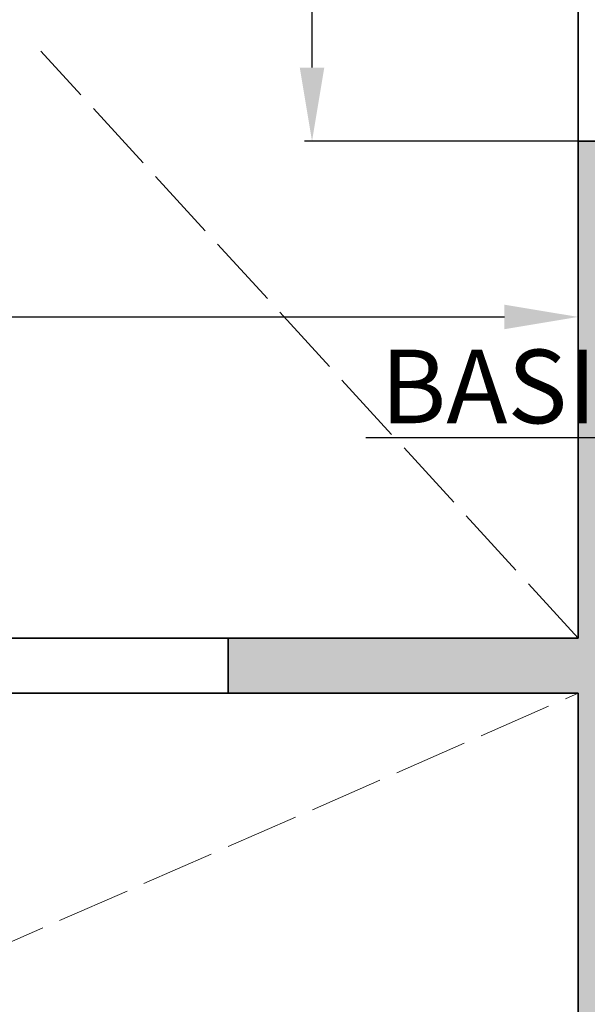
# Model space of a CAD drawing. Units: inches. Extents: x 2083 to 3317, y 1141 to 2115.
# Tile 112 of 256: x 2772 to 2864, y 1361 to 1522. Entities that reach past the tile are written whole.
import ezdxf

# ---------------------------------------------------------------- set-up
doc = ezdxf.new("R2010")
doc.units = ezdxf.units.IN
doc.linetypes.add('ACAD_ISO02W100', pattern=[15, 12, -3])
for name, color, linetype, lineweight in [('A-ANNO-DIMS', 2, 'Continuous', 18), ('A-FLOR-OPEN', 8, 'ACAD_ISO02W100', 13), ('A-WALL', 7, 'Continuous', 35)]:
    doc.layers.add(name, color=color, linetype=linetype, lineweight=lineweight)
doc.layers.add('A-WALL-PATT', color=251, linetype='Continuous', lineweight=13, true_color=0x636466)
doc.styles.get("Standard").update_dxf_attribs({"font": 'arial.ttf'})
doc.dimstyles.new('ISO-25', dxfattribs={"dimtxt": 12, "dimasz": 12, "dimexe": 1.25, "dimexo": 0.625, "dimtad": 1, "dimlunit": 3, "dimtxsty": 'Standard', "dimcen": 2.5, "dimadec": 0, "dimazin": 0, "dimtfac": 1, "dimtmove": 0, "dimatfit": 3, "dimfxl": 1, "dimarcsym": 0})

# ---------------------------------------------------------------- blocks, each defined once
blk = doc.blocks.new('*D18')
at = {"layer": 'A-ANNO-DIMS', "color": 0, "lineweight": -2, "transparency": 16777216}
for p, q in [((3018.48, 1456.16), (3018.48, 1452.14)), ((3041.07, 1456.16), (3041.07, 1452.14)), ((3006.48, 1453.39), (2828.36, 1453.39)), ((3041.07, 1453.39), (3018.48, 1453.39)), ((3053.07, 1453.39), (3065.07, 1453.39))]:
    blk.add_line(p, q, dxfattribs=at)
at = {"layer": 'A-ANNO-DIMS', "color": 0, "transparency": 16777216}
for points in [[(3006.48, 1455.39), (3006.48, 1451.39), (3018.48, 1453.39)], [(3053.07, 1455.39), (3053.07, 1451.39), (3041.07, 1453.39)]]:
    blk.add_solid(points, dxfattribs=at)
at = {"layer": 'Defpoints', "color": 0, "transparency": 16777216}
for p in [(3018.48, 1456.78), (3041.07, 1456.78), (3018.48, 1453.39)]:
    blk.add_point(p, dxfattribs=at)
at = {"layer": 'A-ANNO-DIMS', "color": 0, "transparency": 16777216, "insert": (2911.42, 1460.22), "char_height": 12, "attachment_point": 5}
blk.add_mtext('BASIN 1\'-10 1/2" TYP.', dxfattribs=at)
blk = doc.blocks.new('*D43')
at = {"layer": 'A-ANNO-DIMS', "color": 0, "lineweight": -2, "transparency": 16777216}
for p, q in [((2604.96, 1421.39), (2604.96, 1474.36)), ((2862.96, 1421.39), (2862.96, 1474.36)), ((2616.96, 1473.11), (2850.96, 1473.11))]:
    blk.add_line(p, q, dxfattribs=at)
at = {"layer": 'A-ANNO-DIMS', "color": 0, "transparency": 16777216}
for points in [[(2616.96, 1475.11), (2616.96, 1471.11), (2604.96, 1473.11)], [(2850.96, 1475.11), (2850.96, 1471.11), (2862.96, 1473.11)]]:
    blk.add_solid(points, dxfattribs=at)
at = {"layer": 'Defpoints', "color": 0, "transparency": 16777216}
for p in [(2862.96, 1473.11), (2604.96, 1420.76), (2862.96, 1420.76)]:
    blk.add_point(p, dxfattribs=at)
at = {"layer": 'A-ANNO-DIMS', "color": 0, "transparency": 16777216, "insert": (2733.96, 1479.86), "char_height": 12, "attachment_point": 5}
blk.add_mtext('21\'-6"', dxfattribs=at)
blk = doc.blocks.new('*D57')
at = {"layer": 'A-ANNO-DIMS', "color": 0, "lineweight": -2, "transparency": 16777216}
for p, q in [((2871.33, 1621.76), (2818.36, 1621.76)), ((2819.61, 1513.76), (2819.61, 1609.76)), ((2871.33, 1501.76), (2818.36, 1501.76))]:
    blk.add_line(p, q, dxfattribs=at)
at = {"layer": 'A-ANNO-DIMS', "color": 0, "transparency": 16777216}
for points in [[(2817.61, 1609.76), (2821.61, 1609.76), (2819.61, 1621.76)], [(2817.61, 1513.76), (2821.61, 1513.76), (2819.61, 1501.76)]]:
    blk.add_solid(points, dxfattribs=at)
at = {"layer": 'Defpoints', "color": 0, "transparency": 16777216}
for p in [(2819.61, 1621.76), (2871.96, 1621.76), (2871.96, 1501.76)]:
    blk.add_point(p, dxfattribs=at)
at = {"layer": 'A-ANNO-DIMS', "color": 0, "transparency": 16777216, "insert": (2812.86, 1561.76), "char_height": 12, "attachment_point": 5, "rotation": 90}
blk.add_mtext('10\'-0"', dxfattribs=at)

msp = doc.modelspace()

# ---------------------------------------------------------------- hatches: boundary and pattern name
at = {"layer": 'A-WALL-PATT'}
h = msp.add_hatch(color=256, dxfattribs=at)
h.dxf.hatch_style = 1
h.paths.add_polyline_path([(3126.96, 2020.761), (2748.96, 2020.761), (2604.96, 2020.761), (2226.96, 2020.761), (2226.96, 1702.761), (2466.96, 1702.761), (2466.96, 1582.761), (2418.96, 1582.761), (2418.96, 1477.761), (2226.96, 1477.761), (2226.96, 1263.261), (2544.96, 1263.261), (2544.96, 1411.761), (2604.96, 1411.761), (2685.96, 1411.761), (2685.96, 1420.761), (2604.96, 1420.761), (2604.96, 1573.761), (2604.96, 1702.761), (2604.96, 2011.761), (2748.96, 2011.761), (2748.96, 1702.761), (2862.96, 1702.761), (2862.96, 1621.761), (2871.96, 1621.761), (2871.96, 1702.761), (2883.96, 1702.761), (2883.96, 1706.939, -0.0264593), (2883.96, 1711.761), (2757.96, 1711.761), (2757.96, 1807.761), (2787.96, 1807.761), (2787.96, 1812.261), (2757.96, 1812.261), (2757.96, 2011.761), (2877.96, 2011.761), (2877.96, 1812.261), (2847.96, 1812.261), (2847.96, 1807.761), (2889.836, 1807.761), (2889.836, 1812.261), (2882.46, 1812.261), (2882.46, 2011.761), (3117.96, 2011.761), (3117.96, 1812.261), (2937.836, 1812.261), (2937.836, 1807.761), (2995.71, 1807.761), (2995.71, 1796.118), (3000.21, 1796.118), (3000.21, 1807.761), (3117.96, 1807.761), (3117.96, 1711.761), (3000.21, 1711.761), (3000.21, 1760.118), (2998.573, 1760.118, -0.020711), (2995.71, 1760.118), (2995.71, 1711.761), (2931.96, 1711.761), (2931.96, 1702.761), (3126.96, 1702.761)])
h.paths.add_polyline_path([(2471.46, 2011.761), (2471.46, 1810.011), (2462.717, 1810.011), (2462.717, 1805.511), (2505.96, 1805.511), (2505.96, 1810.011), (2475.96, 1810.011), (2475.96, 2011.761), (2595.96, 2011.761), (2595.96, 1810.011), (2565.96, 1810.011), (2565.96, 1805.511), (2595.96, 1805.511), (2595.96, 1711.761), (2235.96, 1711.761), (2235.96, 1805.511), (2353.71, 1805.511), (2353.71, 1796.054), (2358.21, 1796.054), (2358.21, 1805.511), (2414.717, 1805.511), (2414.717, 1810.011), (2235.96, 1810.011), (2235.96, 2011.761)], flags=16)
h.paths.add_polyline_path([(2270.205, 1994.61), (2270.205, 1970.61), (2246.205, 1970.61), (2246.205, 1994.61)], flags=0)
edge = h.paths.add_edge_path(flags=0)
edge.add_ellipse((2332.027, 1899.798), major_axis=(-3.043, 3.043), ratio=0.1682525, start_angle=-161.33217, end_angle=-156.30711, ccw=False)
edge.add_ellipse((2333.082, 1898.744), major_axis=(-1.055, 1.055), ratio=0.4535321, start_angle=-123.37102, end_angle=-94.15911)
edge = h.paths.add_edge_path(flags=0)
edge.add_ellipse((2332.027, 1968.876), major_axis=(3.043, 3.043), ratio=0.1682525, start_angle=18.66783, end_angle=23.69289)
edge.add_spline(control_points=[(2332.926, 1970.691), (2332.227, 1970.336), (2330.894, 1969.659), (2328.413, 1970.932), (2327.204, 1967.749), (2324.71, 1969.956), (2322.533, 1967.012), (2320.013, 1971.296), (2317.68, 1968.158), (2316.041, 1967.102), (2315.427, 1966.81)], knot_values=[0, 0, 0, 0, 2.2670587, 4.3245589, 6.6855835, 8.8786411, 11.121502, 14.300359, 17.7552837, 19.732645, 19.732645, 19.732645, 19.732645], degree=3, periodic=0)
edge.add_ellipse((2332.027, 1968.876), major_axis=(3.043, 3.043), ratio=0.1682525, start_angle=18.66783, end_angle=23.69289, ccw=False)
edge.add_ellipse((2333.082, 1969.931), major_axis=(1.055, 1.055), ratio=0.4535321, start_angle=56.62898, end_angle=85.84089, ccw=False)
edge = h.paths.add_edge_path(flags=0)
edge.add_spline(control_points=[(2296.428, 1967.988), (2293.628, 1965.336), (2287.704, 1959.727), (2299.744, 1949.996), (2294.533, 1935.669), (2290.573, 1920.604), (2293.394, 1909.974), (2296.185, 1904.967)], knot_values=[0.0991853, 0.0991853, 0.0991853, 0.0991853, 0.3453009, 0.6198217, 0.9826526, 1.3860932, 1.8105546, 1.8105546, 1.8105546, 1.8105546], degree=3, periodic=0)
edge.add_spline(control_points=[(2296.185, 1904.967), (2297.384, 1902.619), (2298.001, 1901.949), (2298.553, 1901.468)], knot_values=[0.0062457, 0.0062457, 0.0062457, 0.0062457, 0.0554759, 0.0554759, 0.0554759, 0.0554759], degree=3, periodic=0)
edge.add_spline(control_points=[(2298.553, 1901.468), (2297.259, 1900.923), (2295.225, 1900.232), (2293.06, 1900.614), (2292.101, 1900.788), (2292.09, 1900.791)], knot_values=[0.3128349, 0.3128349, 0.3128349, 0.3128349, 0.4017797, 0.4749867, 0.4759027, 0.4759027, 0.4759027, 0.4759027], degree=3, periodic=0)
edge.add_arc((2292.794, 1904.664), 3.937, 215.4209, 259.69818, ccw=False)
edge.add_spline(control_points=[(2289.585, 1902.382), (2289.477, 1902.535), (2289.368, 1902.688), (2289.261, 1902.841)], knot_values=[0.1028719, 0.1028719, 0.1028719, 0.1028719, 0.1168958, 0.1168958, 0.1168958, 0.1168958], degree=3, periodic=0)
edge.add_spline(control_points=[(2289.261, 1902.841), (2288.687, 1902.55), (2287.64, 1902.02), (2285.881, 1901.874), (2283.853, 1901.504), (2281.72, 1899.711), (2278.467, 1899.493), (2276.157, 1901.883), (2272.259, 1899.804), (2267.778, 1901.843), (2262.244, 1900.184), (2257.415, 1901.782), (2254.318, 1900.726), (2253.178, 1900.337)], knot_values=[0, 0, 0, 0, 1.9079767, 3.4771759, 5.261074, 7.9728515, 11.6802485, 13.7179214, 16.9395917, 22.789562, 27.5025027, 33.5952153, 37.1456181, 37.1456181, 37.1456181, 37.1456181], degree=3, periodic=0)
edge.add_line((2253.178, 1900.337), (2250.244, 1902.841))
edge.add_line((2250.244, 1902.841), (2250.244, 1965.833))
edge.add_line((2250.244, 1965.833), (2253.178, 1968.337))
edge.add_spline(control_points=[(2253.178, 1968.337), (2254.318, 1967.948), (2257.415, 1966.892), (2262.244, 1968.49), (2267.778, 1966.831), (2271.527, 1968.537), (2273.876, 1967.828), (2274.207, 1967.728)], knot_values=[0, 0, 0, 0, 0.0901802, 0.2449351, 0.3646438, 0.5132331, 0.5378548, 0.5378548, 0.5378548, 0.5378548], degree=3, periodic=0)
edge.add_arc((2274.353, 1963.793), 3.937, 72.05113, 92.12795, ccw=False)
edge.add_arc((2281.297, 1985.23), 18.596, 252.05113, 288.56572)
edge.add_arc((2292.317, 1956.029), 12.646, 71.02679, 113.77822, ccw=False)
edge = h.paths.add_edge_path(flags=0)
edge.add_spline(control_points=[(2274.899, 1951.856), (2275.066, 1951.617), (2275.233, 1951.377), (2275.398, 1951.136)], knot_values=[1.4099157, 1.4099157, 1.4099157, 1.4099157, 1.4315903, 1.4315903, 1.4315903, 1.4315903], degree=3, periodic=0)
edge.add_spline(control_points=[(2275.398, 1951.136), (2275.792, 1950.562), (2276.179, 1949.984), (2276.546, 1949.397)], knot_values=[1.3582378, 1.3582378, 1.3582378, 1.3582378, 1.4099157, 1.4099157, 1.4099157, 1.4099157], degree=3, periodic=0)
edge.add_line((2276.546, 1949.397), (2277.437, 1947.862))
edge.add_spline(control_points=[(2277.437, 1947.862), (2276.304, 1945.673), (2274.64, 1942.427), (2274.632, 1938.094), (2272.799, 1930.852), (2274.356, 1943.897), (2275.948, 1947.923), (2276.546, 1949.397)], knot_values=[0.0056315, 0.0056315, 0.0056315, 0.0056315, 0.1860139, 0.2660015, 0.3570872, 0.5963902, 0.7397317, 0.7397317, 0.7397317, 0.7397317], degree=3, periodic=0)
edge.add_spline(control_points=[(2276.546, 1949.397), (2276.179, 1949.984), (2275.792, 1950.562), (2275.398, 1951.136)], knot_values=[1.3582378, 1.3582378, 1.3582378, 1.3582378, 1.4099157, 1.4099157, 1.4099157, 1.4099157], degree=3, periodic=0)
edge.add_spline(control_points=[(2275.398, 1951.136), (2274.943, 1950.08), (2274.208, 1948.025), (2273.935, 1944.851), (2272.469, 1937.627), (2273.466, 1945.696), (2274.701, 1951.059), (2274.899, 1951.856)], knot_values=[0.1043639, 0.1043639, 0.1043639, 0.1043639, 0.1896363, 0.2696239, 0.3607096, 0.6000126, 0.6446217, 0.6446217, 0.6446217, 0.6446217], degree=3, periodic=0)
h.paths.add_polyline_path([(2269.168, 1963.128, -0.3575267), (2268.171, 1960.976, -0.0925607), (2268.171, 1939.436, -0.3575267), (2269.168, 1937.285, -0.3575267), (2267.016, 1938.282, -0.1647847), (2254.686, 1938.282, -0.3575267), (2252.534, 1937.285, -0.3575267), (2253.531, 1939.436, -0.0925607), (2253.531, 1960.976, -0.3575267), (2252.534, 1963.128, -0.3575267), (2254.686, 1962.131, -0.1647847), (2267.016, 1962.131, -0.3575267)], flags=0)
h.paths.add_polyline_path([(2248.874, 1967.802), (2248.874, 1957.028), (2249.458, 1957.028), (2249.458, 1911.647), (2248.874, 1911.647), (2248.874, 1900.873), (2246.512, 1900.873, 0.1973271), (2244.15, 1902.457), (2244.15, 1966.218, 0.1973271), (2246.512, 1967.802)], flags=0)
h.paths.add_polyline_path([(2269.168, 1931.389, -0.3575267), (2268.171, 1929.238, -0.0925607), (2268.171, 1907.698, -0.3575267), (2269.168, 1905.547, -0.3575267), (2267.016, 1906.544, -0.1647847), (2254.686, 1906.544, -0.3575267), (2252.534, 1905.547, -0.3575267), (2253.531, 1907.698, -0.0925607), (2253.531, 1929.238, -0.3575267), (2252.534, 1931.389, -0.3575267), (2254.686, 1930.392, -0.1647847), (2267.016, 1930.392, -0.3575267)], flags=0)
edge = h.paths.add_edge_path(flags=0)
edge.add_spline(control_points=[(2276.197, 1906.724), (2276.168, 1909.029), (2276.114, 1913.372), (2270.598, 1924.925), (2273.905, 1919.013), (2275.922, 1916.262), (2275.475, 1912.402), (2277.258, 1910.381), (2276.696, 1908.225), (2276.646, 1906.813), (2276.618, 1906.008)], knot_values=[0, 0, 0, 0, 8.6102597, 16.2212739, 18.8430575, 23.8048978, 27.4408283, 29.3561016, 31.2034776, 33.6506866, 33.6506866, 33.6506866, 33.6506866], degree=3, periodic=0)
edge.add_spline(control_points=[(2276.618, 1906.008), (2276.623, 1905.624), (2276.498, 1904.629), (2275.442, 1903.855), (2274.937, 1903.08), (2274.859, 1902.841)], knot_values=[0.1564884, 0.1564884, 0.1564884, 0.1564884, 0.1843975, 0.2313765, 0.2505985, 0.2505985, 0.2505985, 0.2505985], degree=3, periodic=0)
edge.add_line((2274.859, 1902.841), (2276.506, 1902.841))
edge.add_spline(control_points=[(2276.506, 1902.841), (2276.788, 1903.085), (2277.665, 1904.125), (2278.25, 1904.341), (2277.654, 1908.527), (2278.156, 1906.228), (2278.1, 1905.286), (2278.847, 1904.069), (2277.857, 1903.415), (2277.874, 1902.991), (2277.904, 1902.841)], knot_values=[0.0595743, 0.0595743, 0.0595743, 0.0595743, 0.0807529, 0.1037415, 0.1697201, 0.1760361, 0.2071372, 0.2404744, 0.2623409, 0.2736605, 0.2736605, 0.2736605, 0.2736605], degree=3, periodic=0)
edge.add_line((2277.904, 1902.841), (2280.03, 1902.841))
edge.add_spline(control_points=[(2280.03, 1902.841), (2279.888, 1903.088), (2279.499, 1903.982), (2280.152, 1905.939), (2278.104, 1909.658), (2279.762, 1907.185), (2280.328, 1904.875), (2280.485, 1903.49), (2281.463, 1903.249), (2281.758, 1902.936), (2281.834, 1902.841)], knot_values=[0.013856, 0.013856, 0.013856, 0.013856, 0.0348738, 0.0888667, 0.1078792, 0.1267378, 0.158714, 0.1937575, 0.2174868, 0.2267221, 0.2267221, 0.2267221, 0.2267221], degree=3, periodic=0)
edge.add_spline(control_points=[(2281.834, 1902.841), (2281.788, 1902.827), (2281.647, 1902.783), (2281.396, 1902.859), (2281.088, 1902.985), (2280.721, 1903.061), (2280.333, 1903.026), (2280.125, 1902.899), (2280.03, 1902.841)], knot_values=[0, 0, 0, 0, 0.1441304, 0.435517, 0.7492759, 1.1530457, 1.5483707, 1.878348, 1.878348, 1.878348, 1.878348], degree=3, periodic=0)
edge.add_line((2280.03, 1902.841), (2277.904, 1902.841))
edge.add_spline(control_points=[(2277.904, 1902.841), (2277.893, 1902.796), (2277.865, 1902.68), (2277.607, 1902.687), (2277.274, 1902.801), (2276.838, 1902.62), (2276.584, 1902.789), (2276.506, 1902.841)], knot_values=[0, 0, 0, 0, 0.1271885, 0.3261988, 0.6280094, 1.2435704, 1.5153306, 1.5153306, 1.5153306, 1.5153306], degree=3, periodic=0)
edge.add_line((2276.506, 1902.841), (2274.859, 1902.841))
edge.add_spline(control_points=[(2274.859, 1902.841), (2274.814, 1902.899), (2274.725, 1903.013), (2274.493, 1903.119), (2274.244, 1902.961), (2273.937, 1903.185), (2273.614, 1902.983), (2273.408, 1902.883), (2273.322, 1902.841)], knot_values=[0, 0, 0, 0, 0.2184302, 0.4369566, 0.6879766, 0.9903786, 1.3983955, 1.6918498, 1.6918498, 1.6918498, 1.6918498], degree=3, periodic=0)
edge.add_spline(control_points=[(2273.322, 1902.841), (2273.617, 1903.446), (2274.274, 1904.538), (2276.027, 1904.574), (2276.207, 1906.584), (2276.197, 1906.724)], knot_values=[0.0122268, 0.0122268, 0.0122268, 0.0122268, 0.0594721, 0.1062177, 0.134458, 0.134458, 0.134458, 0.134458], degree=3, periodic=0)
h.paths.add_polyline_path([(2270.776, 1897.79), (2270.776, 1873.79), (2246.776, 1873.79), (2246.776, 1897.79)], flags=0)
h.paths.add_polyline_path([(2353.71, 1760.005), (2353.71, 1760.054), (2358.21, 1760.054, -0.033729)], flags=0)
h.paths.add_polyline_path([(2321.819, 1737.529), (2341.995, 1737.529, -0.4142136), (2343.203, 1736.321), (2343.203, 1721.021, -0.4142136), (2341.995, 1719.813), (2321.819, 1719.813, -0.4142136), (2320.611, 1721.021), (2320.611, 1736.321, -0.4142136)], flags=0)
h.paths.add_polyline_path([(2324.235, 1736.321), (2339.579, 1736.321, -0.4142136), (2341.995, 1733.905), (2341.995, 1725.45, -0.4142136), (2339.579, 1723.034), (2333.681, 1723.034), (2333.845, 1722.045, -0.8706461), (2335.425, 1721.826, -0.767327), (2333.923, 1721.423), (2331.291, 1721.423, -0.767327), (2329.788, 1721.826, -0.8706461), (2331.368, 1722.045), (2331.533, 1723.034), (2324.235, 1723.034, -0.4142136), (2321.819, 1725.45), (2321.819, 1733.905, -0.4142136)], flags=0)
h.paths.add_polyline_path([(2570.484, 1928.615), (2589.684, 1928.615), (2590.169, 1928.615), (2590.169, 1904.993), (2570.484, 1904.993)], flags=0)
h.paths.add_polyline_path([(2574.447, 1927.264, -1), (2572.829, 1927.264, -1)], flags=0)
h.paths.add_polyline_path([(2573.09, 1926.941), (2573.925, 1927.776), (2574.148, 1927.553), (2573.313, 1926.718)], flags=0)
h.paths.add_polyline_path([(2578.779, 1919.73, -1), (2571.592, 1919.73, -1)], flags=0)
h.paths.add_polyline_path([(2578.385, 1919.73, -1), (2571.985, 1919.73, -1)], flags=0)
h.paths.add_polyline_path([(2331.596, 1729.476, -1), (2333.618, 1729.476, -1)], flags=0)
h.paths.add_polyline_path([(2578.034, 1927.264, -1), (2576.416, 1927.264, -1)], flags=0)
h.paths.add_polyline_path([(2576.689, 1927.531), (2576.912, 1927.754), (2577.747, 1926.919), (2577.524, 1926.696)], flags=0)
h.paths.add_polyline_path([(2578.139, 1909.86, -1), (2572.232, 1909.86, -1)], flags=0)
h.paths.add_polyline_path([(2577.745, 1909.86, -1), (2572.625, 1909.86, -1)], flags=0)
h.paths.add_polyline_path([(2583.798, 1927.264, -1), (2582.179, 1927.264, -1)], flags=0)
h.paths.add_polyline_path([(2582.719, 1927.754), (2583.554, 1926.919), (2583.331, 1926.696), (2582.496, 1927.531)], flags=0)
h.paths.add_polyline_path([(2582.496, 1927.531), (2582.719, 1927.754), (2583.554, 1926.919), (2583.331, 1926.696)], flags=0)
h.paths.add_polyline_path([(2587.739, 1920.53, -1), (2581.832, 1920.53, -1)], flags=0)
h.paths.add_polyline_path([(2587.345, 1920.53, -1), (2582.225, 1920.53, -1)], flags=0)
h.paths.add_polyline_path([(2587.385, 1927.264, -1), (2585.766, 1927.264, -1)], flags=0)
h.paths.add_polyline_path([(2586.082, 1926.98), (2586.917, 1927.815), (2587.14, 1927.593), (2586.305, 1926.758)], flags=0)
h.paths.add_polyline_path([(2588.379, 1910.66, -1), (2581.192, 1910.66, -1)], flags=0)
h.paths.add_polyline_path([(2587.985, 1910.66, -1), (2581.585, 1910.66, -1)], flags=0)
h.paths.add_polyline_path([(2417.168, 1729.478), (2437.344, 1729.478, -0.4142136), (2438.552, 1728.27), (2438.552, 1712.969, -0.4142136), (2437.344, 1711.761), (2417.168, 1711.761, -0.4142136), (2415.96, 1712.969), (2415.96, 1728.27, -0.4142136)], flags=0)
h.paths.add_polyline_path([(2419.584, 1728.27), (2434.928, 1728.27, -0.4142136), (2437.344, 1725.854), (2437.344, 1717.398, -0.4142136), (2434.928, 1714.983), (2429.029, 1714.983), (2429.194, 1713.994, -0.8706461), (2430.774, 1713.775, -0.767327), (2429.271, 1713.372), (2426.64, 1713.372, -0.767327), (2425.137, 1713.775, -0.8706461), (2426.717, 1713.994), (2426.882, 1714.983), (2419.584, 1714.983, -0.4142136), (2417.168, 1717.398), (2417.168, 1725.854, -0.4142136)], flags=0)
h.paths.add_polyline_path([(2419.584, 1728.27), (2434.928, 1728.27, -0.4142136), (2437.344, 1725.854), (2437.344, 1717.398, -0.4142136), (2434.928, 1714.983), (2429.029, 1714.983), (2428.358, 1719.009), (2427.553, 1719.009), (2426.882, 1714.983), (2419.584, 1714.983, -0.4142136), (2417.168, 1717.398), (2417.168, 1725.854, -0.4142136)], flags=0)
h.paths.add_polyline_path([(2426.944, 1721.425, -1), (2428.967, 1721.425, -1)], flags=0)
h.paths.add_polyline_path([(2475.96, 1702.761), (2595.96, 1702.761), (2595.96, 1582.761), (2475.96, 1582.761)], flags=16)
h.paths.add_polyline_path([(2427.96, 1573.761), (2595.96, 1573.761), (2595.96, 1468.761), (2595.96, 1420.761), (2384.46, 1420.761), (2384.46, 1468.761), (2427.96, 1468.761)], flags=16)
h.paths.add_polyline_path([(2379.96, 1468.761), (2379.96, 1420.761), (2235.96, 1420.761), (2235.96, 1468.761)], flags=16)
h.paths.add_polyline_path([(2317.816, 1466.696), (2337.992, 1466.696, -0.4142136), (2339.2, 1465.488), (2339.2, 1450.187, -0.4142136), (2337.992, 1448.979), (2317.816, 1448.979, -0.4142136), (2316.608, 1450.187), (2316.608, 1465.488, -0.4142136)], flags=0)
h.paths.add_polyline_path([(2320.232, 1465.488), (2335.576, 1465.488, -0.4142136), (2337.992, 1463.072), (2337.992, 1454.616, -0.4142136), (2335.576, 1452.2), (2329.677, 1452.2), (2329.842, 1451.212, -0.8706461), (2331.422, 1450.992, -0.767327), (2329.92, 1450.59), (2327.288, 1450.59, -0.767327), (2325.785, 1450.992, -0.8706461), (2327.365, 1451.212), (2327.53, 1452.2), (2320.232, 1452.2, -0.4142136), (2317.816, 1454.616), (2317.816, 1463.072, -0.4142136)], flags=0)
h.paths.add_polyline_path([(2320.232, 1465.488), (2335.576, 1465.488, -0.4142136), (2337.992, 1463.072), (2337.992, 1454.616, -0.4142136), (2335.576, 1452.2), (2329.677, 1452.2), (2329.006, 1456.227), (2328.201, 1456.227), (2327.53, 1452.2), (2320.232, 1452.2, -0.4142136), (2317.816, 1454.616), (2317.816, 1463.072, -0.4142136)], flags=0)
h.paths.add_polyline_path([(2327.593, 1458.643, -1), (2329.615, 1458.643, -1)], flags=0)
h.paths.add_polyline_path([(2244.412, 1433.34), (2241.921, 1433.34, -0.4142136), (2240.018, 1435.244), (2240.018, 1440.953, -0.4142105), (2241.921, 1442.856), (2244.412, 1442.856, -1.9764724)], flags=0)
h.paths.add_polyline_path([(2245.357, 1434.398, -0.4142136), (2245.357, 1441.799, -2.1440985)], flags=0)
h.paths.add_polyline_path([(2535.96, 1416.261), (2535.96, 1272.261), (2235.96, 1272.261), (2235.96, 1416.261)], flags=16)
h.paths.add_polyline_path([(2260.12, 1384.293), (2260.12, 1362.039), (2237.865, 1362.039), (2237.865, 1384.293)], flags=0)
edge = h.paths.add_edge_path(flags=0)
edge.add_line((2318.252, 1362.093), (2318.146, 1362.001))
edge.add_ellipse((2317.445, 1360.431), major_axis=(2.822, 2.822), ratio=0.1682525, start_angle=18.66783, end_angle=20.94813, ccw=False)
edge.add_ellipse((2318.423, 1361.409), major_axis=(0.978, 0.978), ratio=0.4535321, start_angle=56.62898, end_angle=70.2262, ccw=False)
edge = h.paths.add_edge_path(flags=0)
edge.add_line((2319.107, 1295.571), (2319.015, 1295.677))
edge.add_ellipse((2317.445, 1296.378), major_axis=(-2.822, 2.822), ratio=0.1682525, start_angle=-161.33217, end_angle=-159.05187, ccw=False)
edge.add_ellipse((2318.423, 1295.4), major_axis=(-0.978, 0.978), ratio=0.4535321, start_angle=-123.37102, end_angle=-109.7738)
edge = h.paths.add_edge_path(flags=0)
edge.add_spline(control_points=[(2284.21, 1301.17), (2284.581, 1300.445), (2284.891, 1299.892), (2285.16, 1299.461)], knot_values=[0.0390658, 0.0390658, 0.0390658, 0.0390658, 0.0554759, 0.0554759, 0.0554759, 0.0554759], degree=3, periodic=0)
edge.add_line((2285.16, 1299.461), (2284.21, 1301.17))
edge = h.paths.add_edge_path(flags=0)
edge.add_line((2280.412, 1297.298), (2283.37, 1297.036))
edge.add_line((2283.37, 1297.036), (2286.406, 1297.926))
edge.add_spline(control_points=[(2286.406, 1297.926), (2285.305, 1297.463), (2284.345, 1297.129), (2283.37, 1297.036)], knot_values=[0.3943688, 0.3943688, 0.3943688, 0.3943688, 0.4759027, 0.4759027, 0.4759027, 0.4759027], degree=3, periodic=0)
edge.add_spline(control_points=[(2283.37, 1297.036), (2283.281, 1297.028), (2282.316, 1296.957), (2281.313, 1297.134), (2280.423, 1297.296), (2280.412, 1297.298)], knot_values=[0.3128349, 0.3128349, 0.3128349, 0.3128349, 0.3202458, 0.3934528, 0.3943688, 0.3943688, 0.3943688, 0.3943688], degree=3, periodic=0)
edge = h.paths.add_edge_path(flags=0)
edge.add_line((2284.436, 1359.607), (2280.446, 1355.328))
edge.add_line((2280.446, 1355.328), (2279.58, 1351.018))
edge.add_line((2279.58, 1351.018), (2282.413, 1346.58))
edge.add_spline(control_points=[(2282.413, 1346.58), (2283.153, 1345.589), (2284.253, 1344.029), (2284.801, 1342.387), (2284.935, 1341.806)], knot_values=[1.2400982, 1.2400982, 1.2400982, 1.2400982, 1.3328922, 1.3827123, 1.3827123, 1.3827123, 1.3827123], degree=3, periodic=0)
edge.add_spline(control_points=[(2284.935, 1341.806), (2285.319, 1340.141), (2285.233, 1338.409), (2284.91, 1336.654)], knot_values=[1.0974841, 1.0974841, 1.0974841, 1.0974841, 1.2400982, 1.2400982, 1.2400982, 1.2400982], degree=3, periodic=0)
edge.add_spline(control_points=[(2284.91, 1336.654), (2284.587, 1334.899), (2284.027, 1333.12), (2283.463, 1331.361)], knot_values=[0.9548699, 0.9548699, 0.9548699, 0.9548699, 1.0974841, 1.0974841, 1.0974841, 1.0974841], degree=3, periodic=0)
edge.add_line((2283.463, 1331.361), (2281.89, 1326.153))
edge.add_line((2281.89, 1326.153), (2280.756, 1321.056))
edge.add_line((2280.756, 1321.056), (2280.299, 1316.002))
edge.add_line((2280.299, 1316.002), (2280.716, 1310.95))
edge.add_line((2280.716, 1310.95), (2282.028, 1305.972))
edge.add_line((2282.028, 1305.972), (2284.21, 1301.17))
edge.add_spline(control_points=[(2284.21, 1301.17), (2283.341, 1302.73), (2282.612, 1304.336), (2282.028, 1305.972)], knot_values=[0.0991853, 0.0991853, 0.0991853, 0.0991853, 0.2417994, 0.2417994, 0.2417994, 0.2417994], degree=3, periodic=0)
edge.add_spline(control_points=[(2282.028, 1305.972), (2281.444, 1307.608), (2281.005, 1309.273), (2280.716, 1310.95)], knot_values=[0.2417994, 0.2417994, 0.2417994, 0.2417994, 0.3844135, 0.3844135, 0.3844135, 0.3844135], degree=3, periodic=0)
edge.add_spline(control_points=[(2280.716, 1310.95), (2280.433, 1312.588), (2280.289, 1314.277), (2280.299, 1315.962), (2280.299, 1316.002)], knot_values=[0.3844135, 0.3844135, 0.3844135, 0.3844135, 0.5236467, 0.5270276, 0.5270276, 0.5270276, 0.5270276], degree=3, periodic=0)
edge.add_spline(control_points=[(2280.299, 1316.002), (2280.312, 1317.687), (2280.478, 1319.368), (2280.756, 1321.056)], knot_values=[0.5270276, 0.5270276, 0.5270276, 0.5270276, 0.6696417, 0.6696417, 0.6696417, 0.6696417], degree=3, periodic=0)
edge.add_spline(control_points=[(2280.756, 1321.056), (2281.035, 1322.744), (2281.426, 1324.44), (2281.89, 1326.153)], knot_values=[0.6696417, 0.6696417, 0.6696417, 0.6696417, 0.8122558, 0.8122558, 0.8122558, 0.8122558], degree=3, periodic=0)
edge.add_spline(control_points=[(2281.89, 1326.153), (2282.264, 1327.533), (2282.788, 1329.262), (2283.353, 1331.018), (2283.463, 1331.361)], knot_values=[0.8122558, 0.8122558, 0.8122558, 0.8122558, 0.9270873, 0.9548699, 0.9548699, 0.9548699, 0.9548699], degree=3, periodic=0)
edge.add_line((2283.463, 1331.361), (2284.91, 1336.654))
edge.add_line((2284.91, 1336.654), (2284.935, 1341.806))
edge.add_line((2284.935, 1341.806), (2282.413, 1346.58))
edge.add_spline(control_points=[(2282.413, 1346.58), (2281.275, 1348.104), (2280.078, 1349.57), (2279.58, 1351.018)], knot_values=[1.3827123, 1.3827123, 1.3827123, 1.3827123, 1.5253264, 1.5253264, 1.5253264, 1.5253264], degree=3, periodic=0)
edge.add_spline(control_points=[(2279.58, 1351.018), (2279.443, 1351.415), (2279.136, 1352.857), (2279.735, 1354.29), (2280.446, 1355.328)], knot_values=[1.5253264, 1.5253264, 1.5253264, 1.5253264, 1.564439, 1.6679405, 1.6679405, 1.6679405, 1.6679405], degree=3, periodic=0)
edge.add_spline(control_points=[(2280.446, 1355.328), (2281.426, 1356.758), (2282.931, 1358.183), (2284.436, 1359.607)], knot_values=[1.6679405, 1.6679405, 1.6679405, 1.6679405, 1.8105546, 1.8105546, 1.8105546, 1.8105546], degree=3, periodic=0)
edge.add_arc((2280.623, 1348.518), 11.726, 71.02679, 113.77822)
edge.add_arc((2270.405, 1375.595), 17.244, 252.05113, 288.56572, ccw=False)
edge.add_arc((2263.966, 1355.718), 3.651, 72.05113, 92.12795)
edge.add_arc((2263.966, 1355.718), 3.651, 92.12795, 177.98513)
edge.add_spline(control_points=[(2260.318, 1355.846), (2260.26, 1354.221), (2260.551, 1350.187), (2262.999, 1346.766), (2264.473, 1344.649)], knot_values=[1.4315903, 1.4315903, 1.4315903, 1.4315903, 1.5641438, 1.7706953, 1.7706953, 1.7706953, 1.7706953], degree=3, periodic=0)
edge.add_line((2264.473, 1344.649), (2264.936, 1343.983))
edge.add_spline(control_points=[(2263.801, 1340.248), (2263.843, 1340.514), (2264.067, 1341.756), (2264.513, 1343.002), (2264.935, 1343.981)], knot_values=[0.5365702, 0.5365702, 0.5365702, 0.5365702, 0.5593494, 0.6446217, 0.6446217, 0.6446217, 0.6446217], degree=3, periodic=0)
edge.add_spline(control_points=[(2264.935, 1343.981), (2265.118, 1343.715), (2265.299, 1343.448), (2265.477, 1343.179)], knot_values=[1.3840767, 1.3840767, 1.3840767, 1.3840767, 1.4099157, 1.4099157, 1.4099157, 1.4099157], degree=3, periodic=0)
edge.add_spline(control_points=[(2265.477, 1343.179), (2265.655, 1342.911), (2265.829, 1342.641), (2265.999, 1342.369)], knot_values=[1.3582378, 1.3582378, 1.3582378, 1.3582378, 1.3840767, 1.3840767, 1.3840767, 1.3840767], degree=3, periodic=0)
edge.add_line((2265.999, 1342.369), (2266.826, 1340.946))
edge.add_spline(control_points=[(2266.826, 1340.946), (2268.894, 1337.09), (2271.398, 1325.843), (2270.516, 1310.569), (2275.919, 1301.861), (2277.79, 1299.199)], knot_values=[0.1168958, 0.1168958, 0.1168958, 0.1168958, 0.4729873, 1.0509689, 1.3137934, 1.3137934, 1.3137934, 1.3137934], degree=3, periodic=0)
edge.add_spline(control_points=[(2277.79, 1299.199), (2277.839, 1299.128), (2277.889, 1299.057), (2277.94, 1298.987)], knot_values=[0.1098839, 0.1098839, 0.1098839, 0.1098839, 0.1168958, 0.1168958, 0.1168958, 0.1168958], degree=3, periodic=0)
edge.add_line((2277.94, 1298.987), (2277.789, 1299.199))
edge.add_spline(control_points=[(2277.789, 1299.199), (2277.257, 1298.929), (2276.286, 1298.438), (2275.039, 1298.334), (2274.383, 1298.239), (2274.215, 1298.209)], knot_values=[33.1218702, 33.1218702, 33.1218702, 33.1218702, 35.0290557, 36.5982549, 37.1448269, 37.1448269, 37.1448269, 37.1448269], degree=3, periodic=0)
edge.add_line((2274.215, 1298.209), (2273.073, 1297.893))
edge.add_spline(control_points=[(2273.073, 1297.893), (2272.323, 1297.58), (2271.039, 1296.511), (2269.248, 1296.226), (2268.423, 1296.375)], knot_values=[26.5325843, 26.5325843, 26.5325843, 26.5325843, 29.198919, 31.8391012, 31.8391012, 31.8391012, 31.8391012], degree=3, periodic=0)
edge.add_line((2268.423, 1296.375), (2263.879, 1297.458))
edge.add_spline(control_points=[(2263.879, 1297.458), (2263.556, 1297.359), (2261.86, 1296.839), (2260.239, 1297.282), (2258.933, 1297.516)], knot_values=[15.9195506, 15.9195506, 15.9195506, 15.9195506, 16.9395917, 21.2260675, 21.2260675, 21.2260675, 21.2260675], degree=3, periodic=0)
edge.add_line((2258.933, 1297.516), (2254.055, 1297.329))
edge.add_spline(control_points=[(2254.055, 1297.329), (2253.756, 1297.296), (2252.114, 1297.165), (2250.462, 1297.544), (2249.13, 1297.668)], knot_values=[5.3065169, 5.3065169, 5.3065169, 5.3065169, 6.2764352, 10.6130337, 10.6130337, 10.6130337, 10.6130337], degree=3, periodic=0)
edge.add_line((2249.13, 1297.668), (2244.332, 1296.878))
edge.add_line((2244.332, 1296.878), (2241.611, 1299.199))
edge.add_line((2241.611, 1299.199), (2241.611, 1357.609))
edge.add_line((2241.611, 1357.609), (2244.332, 1359.931))
edge.add_line((2244.332, 1359.931), (2252.729, 1359.543))
edge.add_spline(control_points=[(2252.729, 1359.543), (2252.871, 1359.546), (2253.306, 1359.548), (2253.74, 1359.514), (2254.032, 1359.482)], knot_values=[0.233291, 0.233291, 0.233291, 0.233291, 0.2449351, 0.2689274, 0.2689274, 0.2689274, 0.2689274], degree=3, periodic=0)
edge.add_line((2254.032, 1359.482), (2259.587, 1359.416))
edge.add_spline(control_points=[(2259.587, 1359.416), (2260.677, 1359.629), (2262.073, 1359.897), (2263.524, 1359.459), (2263.83, 1359.366)], knot_values=[0.4225164, 0.4225164, 0.4225164, 0.4225164, 0.5132331, 0.5378548, 0.5378548, 0.5378548, 0.5378548], degree=3, periodic=0)
edge.add_arc((2263.966, 1355.718), 3.651, 72.05113, 92.12795, ccw=False)
edge.add_arc((2270.405, 1375.595), 17.244, 252.05113, 288.56572)
edge.add_arc((2280.623, 1348.518), 11.726, 71.02679, 113.77822, ccw=False)
h.paths.add_polyline_path([(2240.341, 1359.435), (2240.341, 1349.444), (2240.882, 1349.444), (2240.882, 1307.365), (2240.341, 1307.365), (2240.341, 1297.374), (2238.15, 1297.374, 0.1973271), (2235.96, 1298.843), (2235.96, 1357.966, 0.1973271), (2238.15, 1359.435)], flags=0)
h.paths.add_polyline_path([(2259.158, 1355.101, -0.3575267), (2258.233, 1353.106, -0.0925607), (2258.233, 1333.133, -0.3575267), (2259.158, 1331.138, -0.3575267), (2257.163, 1332.062, -0.1647847), (2245.729, 1332.062, -0.3575267), (2243.735, 1331.138, -0.3575267), (2244.659, 1333.133, -0.0925607), (2244.659, 1353.106, -0.3575267), (2243.735, 1355.101, -0.3575267), (2245.729, 1354.176, -0.1647847), (2257.163, 1354.176, -0.3575267)], flags=0)
edge = h.paths.add_edge_path(flags=0)
edge.add_line((2265.999, 1342.369), (2266.826, 1340.946))
edge.add_line((2266.826, 1340.946), (2265.308, 1337.814))
edge.add_line((2265.308, 1337.814), (2264.358, 1334.653))
edge.add_line((2264.358, 1334.653), (2264.262, 1333.8))
edge.add_spline(control_points=[(2264.262, 1333.8), (2264.208, 1333.187), (2264.162, 1332.366), (2264.007, 1331.414), (2263.969, 1331.202)], knot_values=[0.4644442, 0.4644442, 0.4644442, 0.4644442, 0.5166905, 0.5316081, 0.5316081, 0.5316081, 0.5316081], degree=3, periodic=0)
edge.add_spline(control_points=[(2263.969, 1331.202), (2263.775, 1330.119), (2263.424, 1328.791), (2263.257, 1328.531), (2263.234, 1328.515)], knot_values=[0.3726816, 0.3726816, 0.3726816, 0.3726816, 0.4488497, 0.4644442, 0.4644442, 0.4644442, 0.4644442], degree=3, periodic=0)
edge.add_spline(control_points=[(2263.234, 1328.515), (2263.096, 1328.42), (2263.131, 1329.301), (2263.275, 1330.616)], knot_values=[0.2809191, 0.2809191, 0.2809191, 0.2809191, 0.3726816, 0.3726816, 0.3726816, 0.3726816], degree=3, periodic=0)
edge.add_spline(control_points=[(2263.275, 1330.616), (2263.419, 1331.93), (2263.672, 1333.677), (2263.97, 1335.315)], knot_values=[0.1891566, 0.1891566, 0.1891566, 0.1891566, 0.2809191, 0.2809191, 0.2809191, 0.2809191], degree=3, periodic=0)
edge.add_spline(control_points=[(2263.97, 1335.315), (2264.1, 1336.032), (2264.419, 1337.622), (2264.755, 1338.864), (2264.947, 1339.491)], knot_values=[0.097394, 0.097394, 0.097394, 0.097394, 0.1375775, 0.1891566, 0.1891566, 0.1891566, 0.1891566], degree=3, periodic=0)
edge.add_spline(control_points=[(2264.947, 1339.491), (2265.29, 1340.606), (2265.644, 1341.494), (2265.999, 1342.369)], knot_values=[0.0056315, 0.0056315, 0.0056315, 0.0056315, 0.097394, 0.097394, 0.097394, 0.097394], degree=3, periodic=0)
h.paths.add_polyline_path([(2259.158, 1325.671, -0.3575267), (2258.233, 1323.676, -0.0925607), (2258.233, 1303.703, -0.3575267), (2259.158, 1301.708, -0.3575267), (2257.163, 1302.633, -0.1647847), (2245.729, 1302.633, -0.3575267), (2243.735, 1301.708, -0.3575267), (2244.659, 1303.703, -0.0925607), (2244.659, 1323.676, -0.3575267), (2243.735, 1325.671, -0.3575267), (2245.729, 1324.747, -0.1647847), (2257.163, 1324.747, -0.3575267)], flags=0)
edge = h.paths.add_edge_path(flags=0)
edge.add_spline(control_points=[(2261.709, 1317.311), (2261.679, 1317.418), (2261.762, 1317.389), (2262.491, 1316.09), (2262.962, 1315.301)], knot_values=[14.9558607, 14.9558607, 14.9558607, 14.9558607, 16.2212739, 18.6948259, 18.6948259, 18.6948259, 18.6948259], degree=3, periodic=0)
edge.add_spline(control_points=[(2262.962, 1315.301), (2262.99, 1315.254), (2263.702, 1314.067), (2264.349, 1313.127), (2264.73, 1312.164)], knot_values=[18.6948259, 18.6948259, 18.6948259, 18.6948259, 18.8430575, 22.433791, 22.433791, 22.433791, 22.433791], degree=3, periodic=0)
edge.add_spline(control_points=[(2264.73, 1312.164), (2264.876, 1311.796), (2265.177, 1310.77), (2265.143, 1309.559), (2265.248, 1308.824)], knot_values=[22.433791, 22.433791, 22.433791, 22.433791, 23.8048978, 26.1727562, 26.1727562, 26.1727562, 26.1727562], degree=3, periodic=0)
edge.add_line((2265.248, 1308.824), (2265.851, 1307.172))
edge.add_spline(control_points=[(2265.851, 1307.172), (2266.065, 1306.822), (2266.384, 1306.332), (2266.424, 1305.781), (2266.42, 1305.611)], knot_values=[28.0625624, 28.0625624, 28.0625624, 28.0625624, 29.3561016, 29.9117214, 29.9117214, 29.9117214, 29.9117214], degree=3, periodic=0)
edge.add_spline(control_points=[(2266.42, 1305.611), (2266.416, 1305.433), (2266.394, 1305.25), (2266.365, 1305.066)], knot_values=[29.9117214, 29.9117214, 29.9117214, 29.9117214, 30.4978371, 30.4978371, 30.4978371, 30.4978371], degree=3, periodic=0)
edge.add_line((2266.365, 1305.066), (2266.066, 1302.136))
edge.add_spline(control_points=[(2266.066, 1302.136), (2266.071, 1301.78), (2265.998, 1301.2), (2265.663, 1300.759), (2265.509, 1300.586)], knot_values=[0.1564884, 0.1564884, 0.1564884, 0.1564884, 0.1843975, 0.2035434, 0.2035434, 0.2035434, 0.2035434], degree=3, periodic=0)
edge.add_line((2265.509, 1300.586), (2264.435, 1299.199))
edge.add_line((2264.435, 1299.199), (2265.962, 1299.199))
edge.add_line((2265.962, 1299.199), (2267.336, 1301.175))
edge.add_line((2267.336, 1301.175), (2267.312, 1301.986))
edge.add_spline(control_points=[(2267.312, 1301.986), (2267.261, 1302.862), (2267.16, 1303.737), (2267.271, 1303.326)], knot_values=[0.1262286, 0.1262286, 0.1262286, 0.1262286, 0.1666174, 0.1666174, 0.1666174, 0.1666174], degree=3, periodic=0)
edge.add_spline(control_points=[(2267.271, 1303.326), (2267.28, 1303.294), (2267.31, 1303.175), (2267.373, 1302.884), (2267.406, 1302.683), (2267.418, 1302.601)], knot_values=[0.1666174, 0.1666174, 0.1666174, 0.1666174, 0.1697201, 0.1760361, 0.1807647, 0.1807647, 0.1807647, 0.1807647], degree=3, periodic=0)
edge.add_spline(control_points=[(2267.744, 1300.988), (2267.688, 1301.151), (2267.481, 1301.657), (2267.484, 1302.145), (2267.418, 1302.601)], knot_values=[0.1807647, 0.1807647, 0.1807647, 0.1807647, 0.1937665, 0.2201389, 0.2201389, 0.2201389, 0.2201389], degree=3, periodic=0)
edge.add_line((2267.418, 1302.601), (2267.744, 1300.988))
edge.add_spline(control_points=[(2267.744, 1300.988), (2267.832, 1300.732), (2267.932, 1300.31), (2267.555, 1299.975), (2267.429, 1299.829)], knot_values=[0.2201389, 0.2201389, 0.2201389, 0.2201389, 0.2404744, 0.2548903, 0.2548903, 0.2548903, 0.2548903], degree=3, periodic=0)
edge.add_line((2267.429, 1299.829), (2267.258, 1299.199))
edge.add_line((2267.258, 1299.199), (2269.23, 1299.199))
edge.add_spline(control_points=[(2269.23, 1299.199), (2269.099, 1299.429), (2268.843, 1300.016), (2269.012, 1300.916), (2268.947, 1301.661)], knot_values=[0.013856, 0.013856, 0.013856, 0.013856, 0.0348738, 0.0670726, 0.0670726, 0.0670726, 0.0670726], degree=3, periodic=0)
edge.add_line((2268.947, 1301.661), (2268.432, 1303.603))
edge.add_spline(control_points=[(2268.432, 1303.603), (2268.176, 1304.192), (2267.596, 1305.251), (2268.041, 1304.623), (2268.251, 1304.282)], knot_values=[0.0901547, 0.0901547, 0.0901547, 0.0901547, 0.1078792, 0.1202891, 0.1202891, 0.1202891, 0.1202891], degree=3, periodic=0)
edge.add_spline(control_points=[(2268.251, 1304.282), (2268.361, 1304.105), (2269.058, 1302.918), (2269.383, 1301.59), (2269.521, 1300.776), (2269.575, 1300.556)], knot_values=[0.1202891, 0.1202891, 0.1202891, 0.1202891, 0.1267378, 0.158714, 0.1735056, 0.1735056, 0.1735056, 0.1735056], degree=3, periodic=0)
edge.add_line((2269.575, 1300.556), (2270.686, 1299.421))
edge.add_spline(control_points=[(2270.686, 1299.421), (2270.767, 1299.357), (2270.838, 1299.281), (2270.903, 1299.199)], knot_values=[0.2181597, 0.2181597, 0.2181597, 0.2181597, 0.2267221, 0.2267221, 0.2267221, 0.2267221], degree=3, periodic=0)
edge.add_line((2270.937, 1299.193), (2270.903, 1299.199))
edge.add_spline(control_points=[(2270.903, 1299.199), (2270.86, 1299.186), (2270.73, 1299.146), (2270.496, 1299.216), (2270.272, 1299.308), (2270.121, 1299.348), (2270.063, 1299.36)], knot_values=[0.939174, 0.939174, 0.939174, 0.939174, 1.0833044, 1.3746911, 1.6884499, 1.878348, 1.878348, 1.878348, 1.878348], degree=3, periodic=0)
edge.add_line((2270.063, 1299.36), (2269.23, 1299.199))
edge.add_line((2269.23, 1299.199), (2267.258, 1299.199))
edge.add_spline(control_points=[(2267.258, 1299.199), (2267.248, 1299.157), (2267.223, 1299.05), (2266.984, 1299.057), (2266.809, 1299.116), (2266.677, 1299.109), (2266.637, 1299.105)], knot_values=[0.7576653, 0.7576653, 0.7576653, 0.7576653, 0.8848538, 1.0838641, 1.3856747, 1.5153306, 1.5153306, 1.5153306, 1.5153306], degree=3, periodic=0)
edge.add_spline(control_points=[(2266.637, 1299.105), (2266.485, 1299.089), (2266.236, 1299.017), (2266.035, 1299.151), (2265.962, 1299.199)], knot_values=[0, 0, 0, 0, 0.4859051, 0.7576653, 0.7576653, 0.7576653, 0.7576653], degree=3, periodic=0)
edge.add_line((2265.962, 1299.199), (2264.435, 1299.199))
edge.add_line((2264.435, 1299.199), (2263.858, 1299.367))
edge.add_spline(control_points=[(2263.858, 1299.367), (2263.819, 1299.371), (2263.78, 1299.386), (2263.74, 1299.402)], knot_values=[0.8459249, 0.8459249, 0.8459249, 0.8459249, 0.9786272, 0.9786272, 0.9786272, 0.9786272], degree=3, periodic=0)
edge.add_line((2263.722, 1299.396), (2263.01, 1299.199))
edge.add_spline(control_points=[(2263.01, 1299.199), (2263.246, 1299.683), (2263.506, 1300.128), (2263.873, 1300.408)], knot_values=[0.0122268, 0.0122268, 0.0122268, 0.0122268, 0.0529705, 0.0529705, 0.0529705, 0.0529705], degree=3, periodic=0)
edge.add_spline(control_points=[(2263.873, 1300.408), (2263.932, 1300.453), (2264.084, 1300.553), (2264.255, 1300.624), (2264.36, 1300.665)], knot_values=[0.0529705, 0.0529705, 0.0529705, 0.0529705, 0.0594721, 0.0690861, 0.0690861, 0.0690861, 0.0690861], degree=3, periodic=0)
edge.add_line((2264.36, 1300.665), (2265.142, 1301.078))
edge.add_line((2265.142, 1301.078), (2265.676, 1302.8))
edge.add_line((2265.676, 1302.8), (2265.541, 1305.704))
edge.add_line((2265.541, 1305.704), (2264.803, 1309.328))
edge.add_line((2264.803, 1309.328), (2263.041, 1314.092))
edge.add_spline(control_points=[(2263.041, 1314.092), (2262.384, 1315.671), (2261.796, 1316.998), (2261.709, 1317.311)], knot_values=[11.2168955, 11.2168955, 11.2168955, 11.2168955, 14.9558607, 14.9558607, 14.9558607, 14.9558607], degree=3, periodic=0)
h.paths.add_polyline_path([(2871.96, 1416.261), (2895.91, 1416.261), (2895.91, 1420.761), (2871.96, 1420.761), (2871.96, 1501.761), (2862.96, 1501.761), (2862.96, 1420.761), (2805.96, 1420.761), (2805.96, 1411.761), (2862.96, 1411.761), (2862.96, 1263.261), (3126.96, 1263.261), (3126.96, 1411.761), (3126.96, 1486.761), (2943.96, 1486.761), (2943.96, 1477.761), (2967.86, 1477.761), (2967.86, 1420.761), (2943.91, 1420.761), (2943.91, 1416.261), (3117.96, 1416.261), (3117.96, 1420.761), (2972.36, 1420.761), (2972.36, 1477.761), (3117.96, 1477.761), (3117.96, 1420.761), (3117.96, 1272.261), (2871.96, 1272.261)], flags=0)
h.paths.add_polyline_path([(2457.126, 1485.943), (2527.603, 1485.943), (2527.603, 1537.636), (2457.126, 1537.636)], flags=8)
h.paths.add_polyline_path([(2481.005, 1609.982), (2590.766, 1609.982), (2590.766, 1682.003), (2481.005, 1682.003)], flags=8)
h.paths.add_polyline_path([(2483.085, 1729.127), (2553.562, 1729.127), (2553.562, 1780.82), (2483.085, 1780.82)], flags=8)
h = msp.add_hatch(color=256, dxfattribs=at)
h.dxf.hatch_style = 1
h.paths.add_polyline_path([(3126.96, 1486.761), (2943.96, 1486.761), (2943.96, 1477.761), (2967.86, 1477.761), (2967.86, 1420.761), (2943.91, 1420.761), (2943.91, 1416.261), (3117.96, 1416.261), (3117.96, 1420.761), (2972.36, 1420.761), (2972.36, 1477.761), (3117.96, 1477.761), (3117.96, 1420.761), (3117.96, 1272.261), (2871.96, 1272.261), (2871.96, 1416.261), (2895.91, 1416.261), (2895.91, 1420.761), (2871.96, 1420.761), (2871.96, 1501.761), (2862.96, 1501.761), (2862.96, 1420.761), (2805.96, 1420.761), (2805.96, 1411.761), (2862.96, 1411.761), (2862.96, 1263.261), (3126.96, 1263.261), (3126.96, 1411.761)])

# ---------------------------------------------------------------- linework, layer by layer
at = {"layer": 'A-FLOR-OPEN'}
for p, q in [((2862.96, 1420.761), (2775.419, 1516.445)), ((2544.96, 1272.261), (2862.96, 1411.761))]:
    msp.add_line(p, q, dxfattribs=at)
at = {"layer": 'A-WALL'}
for p, q in [((2862.96, 1702.761), (2862.96, 1420.761)), ((2871.96, 1501.761), (2862.96, 1501.761)), ((2604.96, 1420.761), (2862.96, 1420.761)), ((2805.96, 1420.761), (2805.96, 1411.761)), ((2733.96, 1411.761), (2862.96, 1411.761)), ((2862.96, 1411.761), (2862.96, 1263.261))]:
    msp.add_line(p, q, dxfattribs=at)

# ---------------------------------------------------------------- dimensions: what is measured, and where the dimension line sits
at = {"layer": 'A-ANNO-DIMS'}
dim = msp.add_linear_dim(base=(2819.61, 1621.761), p1=(2871.96, 1501.761), p2=(2871.96, 1621.761), angle=90, dimstyle='ISO-25', override={"dimdec": 1, "dimlfac": 1, "dimrnd": 0, "dimzin": 1, "dimdsep": 46, "dimlunit": 4, "dimfrac": 2}, dxfattribs=at)
dim.commit()
dim.dimension.update_dxf_attribs({"geometry": '*D57', "text_midpoint": (2812.858, 1561.761)})
dim = msp.add_linear_dim(base=(3018.476, 1453.392), p1=(3041.068, 1456.781), p2=(3018.476, 1456.781), angle=180, text='BASIN <> TYP.', dimstyle='ISO-25', override={"dimdec": 1, "dimlfac": 1, "dimrnd": 0, "dimzin": 1, "dimdsep": 46, "dimlunit": 4, "dimfrac": 2}, dxfattribs=at)
dim.commit()
dim.dimension.update_dxf_attribs({"geometry": '*D18', "text_midpoint": (2911.418, 1460.222)})
dim = msp.add_linear_dim(base=(2862.96, 1473.111), p1=(2604.96, 1420.761), p2=(2862.96, 1420.761), dimstyle='ISO-25', override={"dimdec": 1, "dimlfac": 1, "dimrnd": 0, "dimzin": 1, "dimdsep": 46, "dimlunit": 4, "dimfrac": 2}, dxfattribs=at)
dim.commit()
dim.dimension.update_dxf_attribs({"geometry": '*D43', "text_midpoint": (2733.96, 1479.863)})

doc.saveas('drawing.dxf')
